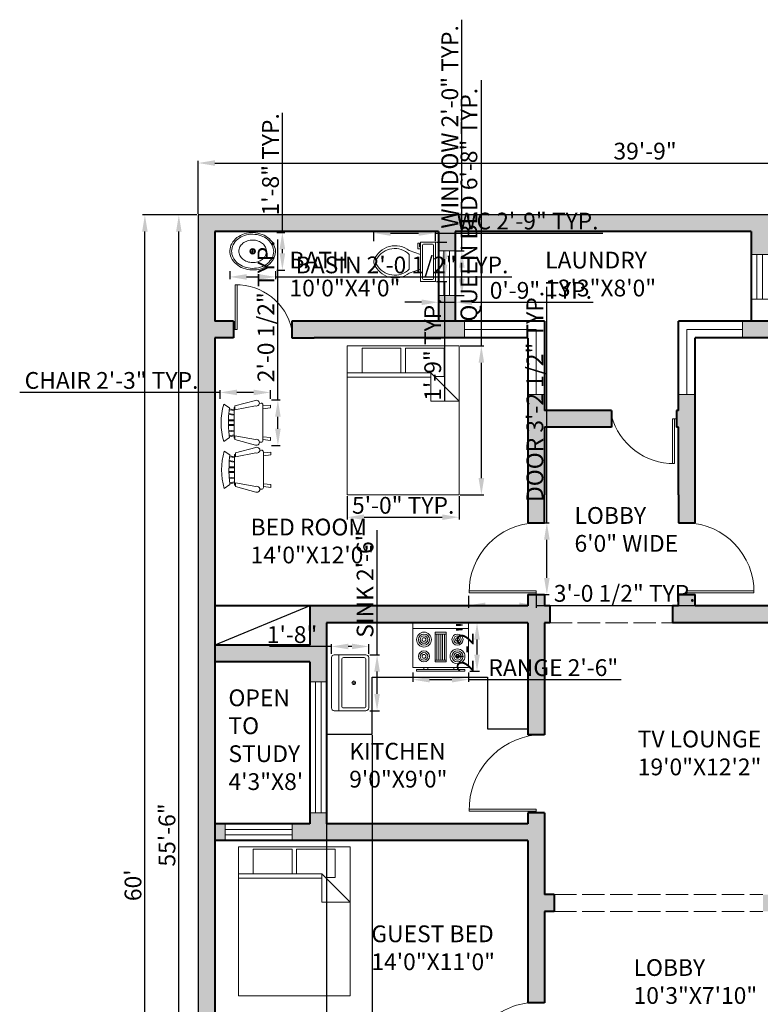
# Model space of a CAD drawing. Units: inches. Extents: x 1967493 to 1968177, y 907234 to 908105.
# Tile 4 of 5: x 1967493 to 1967891, y 907576 to 908105. Entities that reach past the tile are written whole.
import ezdxf

# ---------------------------------------------------------------- set-up
doc = ezdxf.new("R2010")
doc.units = ezdxf.units.IN
doc.linetypes.add('ACAD_ISO02W100', pattern=[15, 12, -3])
for name, color, linetype, lineweight in [('A-ANNO-DIMS', 2, 'Continuous', 18), ('A-AREA-IDEN', 7, 'Continuous', 25), ('A-DOOR', 3, 'Continuous', 20), ('A-EQPM', 8, 'Continuous', 20), ('A-FLOR-CASE', 9, 'Continuous', 25), ('A-FLOR-FIXT', 9, 'Continuous', 18), ('A-FURN', 8, 'Continuous', 18), ('A-GLAZ', 4, 'Continuous', 18), ('A-WALL', 7, 'Continuous', 40), ('A-WALL-OVHD', 7, 'ACAD_ISO02W100', 18), ('C-PROP', 7, 'Continuous', 25)]:
    doc.layers.add(name, color=color, linetype=linetype, lineweight=lineweight)
doc.layers.add('A-WALL-PATT', color=18, linetype='Continuous', lineweight=13, true_color=0x000000)
doc.styles.get("Standard").update_dxf_attribs({"font": 'arial.ttf'})
doc.dimstyles.new('ISO-25', dxfattribs={"dimtxt": 9, "dimasz": 9, "dimexe": 1.25, "dimexo": 0.625, "dimtad": 1, "dimdec": 1, "dimrnd": 9, "dimlunit": 3, "dimtxsty": 'Standard', "dimcen": 2.5, "dimadec": 0, "dimazin": 0, "dimtfac": 1, "dimtdec": 1, "dimtmove": 0, "dimatfit": 3, "dimfxl": 1, "dimarcsym": 0})

# ---------------------------------------------------------------- blocks, each defined once
blk = doc.blocks.new('Bed - Queen')
for p, q in [((0, -80.00003), (0, 0)), ((0, 0), (59.99999, 0)), ((59.99999, 0), (59.99999, -80.00003)), ((7.99999, -1.2), (28.79998, -1.2)), ((7.99999, -14.4), (7.99999, -1.2)), ((28.79998, -1.2), (28.79998, -14.4)), ((31.19999, -1.2), (51.99999, -1.2)), ((31.19999, -14.4), (31.19999, -1.2)), ((51.99999, -1.2), (51.99999, -16.4)), ((0, -14.4), (44.8, -14.4)), ((59.99999, -29.6), (44.8, -14.4)), ((44.8, -14.4), (44.8, -29.6)), ((44.8, -16.8), (0, -16.8)), ((51.99999, -16.4), (46.79936, -16.4)), ((44.8, -29.6), (59.99999, -29.6)), ((59.99999, -80.00003), (0, -80.00003))]:
    blk.add_line(p, q)
blk = doc.blocks.new('Sink - Oval top')
for p, q in [((-1, 0), (1, 0)), ((0, 1), (0, -1))]:
    blk.add_line(p, q)
for points in [[(-12.23, 0.39, 0.117634), (-11.46, -3.36, 0.104469), (-8.88, -6.8, 0.090016), (-5.08, -9.07, 0.08192), (-0.32, -10.02, 0.08192), (4.49, -9.38, 0.090016), (8.42, -7.36, 0.104469), (11.22, -4.09, 0.117634), (12.23, -0.39, 0.117634), (11.46, 3.36, 0.104469), (8.88, 6.8, 0.090016), (5.08, 9.07, 0.08192), (0.32, 10.02, 0.08192), (-4.49, 9.38, 0.090016), (-8.42, 7.36, 0.104469), (-11.22, 4.09, 0.117634)], [(-11.29, 0.16, 0.118622), (-10.52, -3.25, 0.104678), (-8.07, -6.36, 0.089562), (-4.54, -8.37, 0.081185), (-0.13, -9.15, 0.081185), (4.3, -8.49, 0.089562), (7.89, -6.58, 0.104678), (10.42, -3.55, 0.118622), (11.29, -0.16, 0.118622), (10.52, 3.25, 0.104678), (8.07, 6.36, 0.089562), (4.54, 8.37, 0.081185), (0.13, 9.15, 0.081185), (-4.3, 8.49, 0.089562), (-7.89, 6.58, 0.104678), (-10.42, 3.55, 0.118622)], [(-7.42, 0.08, 0.118283), (-6.91, -2.17, 0.104607), (-5.29, -4.21, 0.089718), (-2.97, -5.53, 0.081436), (-0.07, -6.04, 0.081436), (2.84, -5.59, 0.089718), (5.2, -4.33, 0.104607), (6.86, -2.32, 0.118283), (7.42, -0.08, 0.118283), (6.91, 2.17, 0.104607), (5.29, 4.21, 0.089718), (2.97, 5.53, 0.081436), (0.07, 6.04, 0.081436), (-2.84, 5.59, 0.089718), (-5.2, 4.33, 0.104607), (-6.86, 2.32, 0.118283)]]:
    blk.add_lwpolyline(points, format="xyb", close=True)
for radius in [1.5, 1]:
    blk.add_circle((0, 0), radius)
blk = doc.blocks.new('Range-Oven - 30 in top')
for p, q in [((0, -3), (30, -3)), ((12, -6), (18, -6)), ((13, -20), (13, -6)), ((14, -6), (14, -20)), ((15, -20), (15, -6)), ((16, -6), (16, -20)), ((17, -20), (17, -6)), ((18, -20), (12, -20)), ((6, -24), (6, -25)), ((8, -25), (8, -24)), ((22, -25), (22, -24)), ((24, -24), (24, -25))]:
    blk.add_line(p, q)
for points in [[(0, -24), (0, 0), (30, 0), (30, -24)], [(12, -21), (12, -5), (18, -5), (18, -21)], [(2, -26), (2, -25), (28, -25), (28, -26)]]:
    blk.add_lwpolyline(points, close=True)
for centre, radius in [((6, -9), 4), ((6, -9), 3), ((6, -9), 2), ((6, -9), 1), ((24, -9), 3), ((24, -9), 2), ((24, -9), 1), ((6, -18), 3), ((24, -18), 4), ((24, -18), 3), ((6, -18), 2), ((6, -18), 1), ((24, -18), 2), ((24, -18), 1)]:
    blk.add_circle(centre, radius)
blk = doc.blocks.new('Sink-single - 30 in top')
blk.add_line((-15, -3.999996), (15, -3.999996))
for points in [[(-13.5, 0), (13.5, 0)], [(-15, -18.499996), (-15, -1.5)], [(15, -1.5), (15, -18.499996)], [(-13.5, -17.499996), (-13.5, -6.499996)], [(-12.5, -5.499996), (12.5, -5.499996)], [(13.5, -6.499996), (13.5, -17.499996)], [(13.5, -19.999996), (-13.5, -19.999996)], [(12.5, -18.499996), (-12.5, -18.499996)]]:
    blk.add_lwpolyline(points)
for radius in [1, 0.5]:
    blk.add_circle((0, -11.999996), radius)
for centre, radius, start, end in [((-13.5, -1.5), 1.5, 90, 180), ((13.5, -1.5), 1.5, 0, 90), ((-12.5, -6.499996), 1, 90, 180), ((12.5, -6.499996), 1, 0, 90), ((-13.5, -18.499996), 1.5, 180, 270), ((-12.5, -17.499996), 1, 180, 270), ((12.5, -17.499996), 1, 270, 0), ((13.5, -18.499996), 1.5, 270, 0)]:
    blk.add_arc(centre, radius, start, end)
blk = doc.blocks.new('Toilet - top')
for p, q in [((9.5, -6), (9.5, -2)), ((-10, -8.5), (-8, -8.5)), ((-10, -9.5), (-10, -8.5)), ((-7, -9.5), (-10, -9.5)), ((-8, -8.5), (-8, -8)), ((-7, -8), (-7, -9.5)), ((-4, -8), (-6, -14)), ((4, -8), (6, -14)), ((4, -14), (-4, -14))]:
    blk.add_line(p, q)
blk.add_lwpolyline([(10.5, -8), (10.5, 0), (-10.5, 0), (-10.5, -8)], close=True)
for points in [[(-9.5, -2), (-9.5, -6)], [(8.5, -1), (-8.5, -1)], [(-8.5, -7), (8.5, -7)]]:
    blk.add_lwpolyline(points)
for centre, radius, start, end in [((-8.62, -1.88), 0.884, 81.8699, 188.1301), ((8.62, -1.88), 0.884, 351.8699, 98.1301), ((-8.62, -6.12), 0.884, 171.8699, 278.1301), ((8.62, -6.12), 0.884, 261.8699, 8.1301), ((3.52, -21.58), 12.17, 141.4691, 247.9714), ((4.2, -21.82), 11.33, 136.3677, 238.9468), ((-3.52, -21.58), 12.17, 292.0284, 38.5307), ((-4.2, -21.82), 11.33, 301.053, 43.6321), ((0, -27.88), 4, 245.7318, 294.2682), ((0, -29), 4, 254.8605, 285.1395)]:
    blk.add_arc(centre, radius, start, end)
blk = doc.blocks.new('Chair - Rocking')
for p, q in [((-8, -4.5), (-10, -1.5)), ((-7.5, -4.5), (-7, -7)), ((-6.5, -7), (-7.02225, -4.43)), ((-4.5, -7), (-4.96674, -4.19951)), ((-4, -7), (-4.40532, -4.16272)), ((-1.5, -4.05012), (-1.5, -7)), ((-1, -7), (-1, -4.05012)), ((1, -7), (1, -4.04655)), ((1.5, -4.05012), (1.5, -7)), ((4, -7), (4.40187, -4.18694)), ((4.5, -7), (4.96761, -4.19437)), ((6.5, -7), (7, -4.4057)), ((7.5, -4.5), (7, -7)), ((8, -4.5), (10, -1.5)), ((-9, -7.5), (-12, -18.49999)), ((-7, -7.5), (-9, -7.5)), ((-9, -18.49999), (-7, -7.5)), ((-8.23428, -6.99939), (-8.3093, -7.47958)), ((-8.23041, -7), (8.23915, -7)), ((7, -7.5), (9, -7.5)), ((9, -18.49999), (7, -7.5)), ((8.31071, -7.48854), (8.23449, -7.00073)), ((9, -7.5), (12, -18.49999)), ((-10.36644, -20.64523), (-10.5, -21.49999)), ((10.5, -21.49999), (10.3575, -20.58798)), ((-9, -22.49999), (-9.5, -26.49999)), ((0, -22.49999), (-9.5, -22.49999)), ((-8, -26.49999), (-7.5, -22.49999)), ((0, -22.49999), (9.5, -22.49999)), ((8, -26.49999), (7.5, -22.49999)), ((9, -22.49999), (9.5, -26.49999)), ((-9.5, -26.49999), (-8, -26.49999)), ((9.5, -26.49999), (8, -26.49999))]:
    blk.add_line(p, q)
for centre, radius, start, end in [((0, -34.08333), 34.08333, 72.93847, 107.0615), ((0, -68.25004), 64.25, 93.92211, 97.15267), ((0, -68.25004), 64.25, 82.84733, 93.92211), ((-10.5, -18.99999), 1.58114, 161.5651, 18.43495), ((10.5, -18.99999), 1.58114, 161.5651, 18.43495), ((-9.5, -21.49999), 1, 180, 270), ((9.5, -21.49999), 1, 270, 0)]:
    blk.add_arc(centre, radius, start, end)
blk = doc.blocks.new('*D11')
at = {"layer": 'A-ANNO-DIMS', "color": 0, "lineweight": -2, "transparency": 16777216}
for p, q in [((1967588.78, 908000.79), (1967588.78, 908029.28)), ((1967597.78, 908028.03), (1968059.78, 908028.03)), ((1968068.78, 908000.79), (1968068.78, 908029.28))]:
    blk.add_line(p, q, dxfattribs=at)
at = {"layer": 'A-ANNO-DIMS', "color": 0, "transparency": 16777216}
for points in [[(1967597.78, 908029.53), (1967597.78, 908026.53), (1967588.78, 908028.03)], [(1968059.78, 908029.53), (1968059.78, 908026.53), (1968068.78, 908028.03)]]:
    blk.add_solid(points, dxfattribs=at)
at = {"layer": 'Defpoints', "color": 0, "transparency": 16777216}
for p in [(1968068.78, 908028.03), (1967588.78, 908000.17), (1968068.78, 908000.17)]:
    blk.add_point(p, dxfattribs=at)
at = {"layer": 'A-ANNO-DIMS', "color": 0, "transparency": 16777216, "insert": (1967828.78, 908033.25), "char_height": 9, "attachment_point": 5}
blk.add_mtext('39\'-9"', dxfattribs=at)
blk = doc.blocks.new('*D12')
at = {"layer": 'A-ANNO-DIMS', "color": 0, "lineweight": -2, "transparency": 16777216}
for p, q in [((1967588.15, 908000.17), (1967558.93, 908000.17)), ((1967560.18, 907289.17), (1967560.18, 907991.17)), ((1967588.15, 907280.17), (1967558.93, 907280.17))]:
    blk.add_line(p, q, dxfattribs=at)
at = {"layer": 'A-ANNO-DIMS', "color": 0, "transparency": 16777216}
for points in [[(1967558.68, 907991.17), (1967561.68, 907991.17), (1967560.18, 908000.17)], [(1967558.68, 907289.17), (1967561.68, 907289.17), (1967560.18, 907280.17)]]:
    blk.add_solid(points, dxfattribs=at)
at = {"layer": 'Defpoints', "color": 0, "transparency": 16777216}
for p in [(1967560.18, 908000.17), (1967588.78, 908000.17), (1967588.78, 907280.17)]:
    blk.add_point(p, dxfattribs=at)
at = {"layer": 'A-ANNO-DIMS', "color": 0, "transparency": 16777216, "insert": (1967554.96, 907640.17), "char_height": 9, "attachment_point": 5, "rotation": 90}
blk.add_mtext("60'", dxfattribs=at)
blk = doc.blocks.new('*D13')
at = {"layer": 'A-ANNO-DIMS', "color": 0, "lineweight": -2, "transparency": 16777216}
for p, q in [((1967588.15, 908000.17), (1967577.16, 908000.17)), ((1967578.41, 907343.17), (1967578.41, 907991.17)), ((1967588.15, 907334.17), (1967577.16, 907334.17))]:
    blk.add_line(p, q, dxfattribs=at)
at = {"layer": 'A-ANNO-DIMS', "color": 0, "transparency": 16777216}
for points in [[(1967576.91, 907991.17), (1967579.91, 907991.17), (1967578.41, 908000.17)], [(1967576.91, 907343.17), (1967579.91, 907343.17), (1967578.41, 907334.17)]]:
    blk.add_solid(points, dxfattribs=at)
at = {"layer": 'Defpoints', "color": 0, "transparency": 16777216}
for p in [(1967578.41, 908000.17), (1967588.78, 908000.17), (1967588.78, 907334.17)]:
    blk.add_point(p, dxfattribs=at)
at = {"layer": 'A-ANNO-DIMS', "color": 0, "transparency": 16777216, "insert": (1967573.19, 907667.17), "char_height": 9, "attachment_point": 5, "rotation": 90}
blk.add_mtext('55\'-6"', dxfattribs=at)
blk = doc.blocks.new('WIN-36IN')
for p, q in [((0, 9), (0, 0)), ((36, 6), (0, 6)), ((36, 9), (36, 0)), ((36, 3), (0, 3))]:
    blk.add_line(p, q)
blk = doc.blocks.new('DOOR-SINGLE-36IN')
for p, q in [((0, 1), (0, 2)), ((0, 2), (36, 2)), ((36, 1), (0, 1)), ((36, 2), (36, 1)), ((36, 0), (36, 1))]:
    blk.add_line(p, q)
blk.add_arc((37.01, 1.5), 37.01, 91.5627, 180.774)
blk = doc.blocks.new('WIN-24IN')
for p, q in [((0, 24), (9, 24)), ((3, 24), (3, 0)), ((6, 24), (6, 0)), ((0, 0), (9, 0))]:
    blk.add_line(p, q)
blk = doc.blocks.new('*D18')
at = {"layer": 'A-ANNO-DIMS', "color": 0, "lineweight": -2, "transparency": 16777216}
for p, q in [((1967600.56, 907904.83), (1967492.95, 907904.83)), ((1967600.56, 907901.4), (1967600.56, 907906.08)), ((1967618.56, 907904.83), (1967609.56, 907904.83)), ((1967627.56, 907901.4), (1967627.56, 907906.08))]:
    blk.add_line(p, q, dxfattribs=at)
at = {"layer": 'A-ANNO-DIMS', "color": 0, "transparency": 16777216}
for points in [[(1967609.56, 907906.33), (1967609.56, 907903.33), (1967600.56, 907904.83)], [(1967618.56, 907906.33), (1967618.56, 907903.33), (1967627.56, 907904.83)]]:
    blk.add_solid(points, dxfattribs=at)
at = {"layer": 'Defpoints', "color": 0, "transparency": 16777216}
for p in [(1967600.56, 907904.83), (1967600.56, 907900.78), (1967627.56, 907900.78)]:
    blk.add_point(p, dxfattribs=at)
at = {"layer": 'A-ANNO-DIMS', "color": 0, "transparency": 16777216, "insert": (1967542.26, 907910.11), "char_height": 9, "attachment_point": 5}
blk.add_mtext('CHAIR 2\'-3" TYP.', dxfattribs=at)
blk = doc.blocks.new('*D19')
at = {"layer": 'A-ANNO-DIMS', "color": 0, "lineweight": -2, "transparency": 16777216}
for p, q in [((1967631.61, 907900.78), (1967631.61, 907987.01)), ((1967628.19, 907900.78), (1967632.86, 907900.78)), ((1967631.61, 907885.34), (1967631.61, 907891.78)), ((1967628.19, 907876.34), (1967632.86, 907876.34))]:
    blk.add_line(p, q, dxfattribs=at)
at = {"layer": 'A-ANNO-DIMS', "color": 0, "transparency": 16777216}
for points in [[(1967630.11, 907891.78), (1967633.11, 907891.78), (1967631.61, 907900.78)], [(1967630.11, 907885.34), (1967633.11, 907885.34), (1967631.61, 907876.34)]]:
    blk.add_solid(points, dxfattribs=at)
at = {"layer": 'Defpoints', "color": 0, "transparency": 16777216}
for p in [(1967627.56, 907900.78), (1967631.61, 907900.78), (1967627.56, 907876.34)]:
    blk.add_point(p, dxfattribs=at)
at = {"layer": 'A-ANNO-DIMS', "color": 0, "transparency": 16777216, "insert": (1967626.34, 907948.39), "char_height": 9, "attachment_point": 5, "rotation": 90}
blk.add_mtext('2\'-0 1/2" TYP.', dxfattribs=at)
blk = doc.blocks.new('*D24')
at = {"layer": 'A-ANNO-DIMS', "color": 0, "lineweight": -2, "transparency": 16777216}
for p, q in [((1967740.89, 907929.81), (1967740.89, 908072.45)), ((1967729.52, 907929.81), (1967742.14, 907929.81)), ((1967740.89, 907858.81), (1967740.89, 907920.81)), ((1967729.52, 907849.81), (1967742.14, 907849.81))]:
    blk.add_line(p, q, dxfattribs=at)
at = {"layer": 'A-ANNO-DIMS', "color": 0, "transparency": 16777216}
for points in [[(1967739.39, 907920.81), (1967742.39, 907920.81), (1967740.89, 907929.81)], [(1967739.39, 907858.81), (1967742.39, 907858.81), (1967740.89, 907849.81)]]:
    blk.add_solid(points, dxfattribs=at)
at = {"layer": 'Defpoints', "color": 0, "transparency": 16777216}
for p in [(1967728.89, 907929.81), (1967740.89, 907929.81), (1967728.89, 907849.81)]:
    blk.add_point(p, dxfattribs=at)
at = {"layer": 'A-ANNO-DIMS', "color": 0, "transparency": 16777216, "insert": (1967735.34, 908005.63), "char_height": 9, "attachment_point": 5, "rotation": 90}
blk.add_mtext('QUEEN BED 6\'-8" TYP.', dxfattribs=at)
blk = doc.blocks.new('*D25')
at = {"layer": 'A-ANNO-DIMS', "color": 0, "lineweight": -2, "transparency": 16777216}
for p, q in [((1967668.89, 907849.18), (1967668.89, 907836.56)), ((1967728.89, 907849.18), (1967728.89, 907836.56)), ((1967677.89, 907837.81), (1967719.89, 907837.81))]:
    blk.add_line(p, q, dxfattribs=at)
at = {"layer": 'A-ANNO-DIMS', "color": 0, "transparency": 16777216}
for points in [[(1967677.89, 907839.31), (1967677.89, 907836.31), (1967668.89, 907837.81)], [(1967719.89, 907839.31), (1967719.89, 907836.31), (1967728.89, 907837.81)]]:
    blk.add_solid(points, dxfattribs=at)
at = {"layer": 'Defpoints', "color": 0, "transparency": 16777216}
for p in [(1967668.89, 907849.81), (1967728.89, 907849.81), (1967728.89, 907837.81)]:
    blk.add_point(p, dxfattribs=at)
at = {"layer": 'A-ANNO-DIMS', "color": 0, "transparency": 16777216, "insert": (1967698.89, 907843.03), "char_height": 9, "attachment_point": 5}
blk.add_mtext('5\'-0" TYP.', dxfattribs=at)
blk = doc.blocks.new('*D26')
at = {"layer": 'A-ANNO-DIMS', "color": 0, "lineweight": -2, "transparency": 16777216}
for p, q in [((1967683.13, 907986.09), (1967683.13, 907991.67)), ((1967692.13, 907990.42), (1967707.18, 907990.42)), ((1967716.18, 907986.09), (1967716.18, 907991.67)), ((1967716.18, 907990.42), (1967806.1, 907990.42))]:
    blk.add_line(p, q, dxfattribs=at)
at = {"layer": 'A-ANNO-DIMS', "color": 0, "transparency": 16777216}
for points in [[(1967692.13, 907991.92), (1967692.13, 907988.92), (1967683.13, 907990.42)], [(1967707.18, 907991.92), (1967707.18, 907988.92), (1967716.18, 907990.42)]]:
    blk.add_solid(points, dxfattribs=at)
at = {"layer": 'Defpoints', "color": 0, "transparency": 16777216}
for p in [(1967716.18, 907990.42), (1967683.13, 907985.46), (1967716.18, 907985.46)]:
    blk.add_point(p, dxfattribs=at)
at = {"layer": 'A-ANNO-DIMS', "color": 0, "transparency": 16777216, "insert": (1967765.64, 907995.7), "char_height": 9, "attachment_point": 5}
blk.add_mtext('WC 2\'-9" TYP.', dxfattribs=at)
blk = doc.blocks.new('*D27')
at = {"layer": 'A-ANNO-DIMS', "color": 0, "lineweight": -2, "transparency": 16777216}
for p, q in [((1967716.8, 907985.46), (1967722.39, 907985.46)), ((1967721.14, 907976.46), (1967721.14, 907973.46)), ((1967716.8, 907964.46), (1967722.39, 907964.46)), ((1967721.14, 907964.46), (1967721.14, 907900.2))]:
    blk.add_line(p, q, dxfattribs=at)
at = {"layer": 'A-ANNO-DIMS', "color": 0, "transparency": 16777216}
for points in [[(1967719.64, 907976.46), (1967722.64, 907976.46), (1967721.14, 907985.46)], [(1967719.64, 907973.46), (1967722.64, 907973.46), (1967721.14, 907964.46)]]:
    blk.add_solid(points, dxfattribs=at)
at = {"layer": 'Defpoints', "color": 0, "transparency": 16777216}
for p in [(1967716.18, 907985.46), (1967716.18, 907964.46), (1967721.14, 907964.46)]:
    blk.add_point(p, dxfattribs=at)
at = {"layer": 'A-ANNO-DIMS', "color": 0, "transparency": 16777216, "insert": (1967715.92, 907927.83), "char_height": 9, "attachment_point": 5, "rotation": 90}
blk.add_mtext('1\'-9" TYP.', dxfattribs=at)
blk = doc.blocks.new('*D28')
at = {"layer": 'A-ANNO-DIMS', "color": 0, "lineweight": -2, "transparency": 16777216}
for p, q in [((1967605.78, 907969.92), (1967605.78, 907965.61)), ((1967630.33, 907969.92), (1967630.33, 907965.61)), ((1967614.78, 907966.86), (1967621.33, 907966.86)), ((1967630.33, 907966.86), (1967757.24, 907966.86))]:
    blk.add_line(p, q, dxfattribs=at)
at = {"layer": 'A-ANNO-DIMS', "color": 0, "transparency": 16777216}
for points in [[(1967614.78, 907968.36), (1967614.78, 907965.36), (1967605.78, 907966.86)], [(1967621.33, 907968.36), (1967621.33, 907965.36), (1967630.33, 907966.86)]]:
    blk.add_solid(points, dxfattribs=at)
at = {"layer": 'Defpoints', "color": 0, "transparency": 16777216}
for p in [(1967605.78, 907970.55), (1967630.33, 907970.55), (1967630.33, 907966.86)]:
    blk.add_point(p, dxfattribs=at)
at = {"layer": 'A-ANNO-DIMS', "color": 0, "transparency": 16777216, "insert": (1967698.28, 907972.14), "char_height": 9, "attachment_point": 5}
blk.add_mtext('BASIN 2\'-0 1/2" TYP.', dxfattribs=at)
blk = doc.blocks.new('*D29')
at = {"layer": 'A-ANNO-DIMS', "color": 0, "lineweight": -2, "transparency": 16777216}
for p, q in [((1967634.01, 907990.68), (1967634.01, 908054.95)), ((1967630.96, 907990.68), (1967635.26, 907990.68)), ((1967634.01, 907979.55), (1967634.01, 907981.68)), ((1967630.96, 907970.55), (1967635.26, 907970.55))]:
    blk.add_line(p, q, dxfattribs=at)
at = {"layer": 'A-ANNO-DIMS', "color": 0, "transparency": 16777216}
for points in [[(1967632.51, 907981.68), (1967635.51, 907981.68), (1967634.01, 907990.68)], [(1967632.51, 907979.55), (1967635.51, 907979.55), (1967634.01, 907970.55)]]:
    blk.add_solid(points, dxfattribs=at)
at = {"layer": 'Defpoints', "color": 0, "transparency": 16777216}
for p in [(1967630.33, 907990.68), (1967634.01, 907990.68), (1967630.33, 907970.55)]:
    blk.add_point(p, dxfattribs=at)
at = {"layer": 'A-ANNO-DIMS', "color": 0, "transparency": 16777216, "insert": (1967628.79, 908027.31), "char_height": 9, "attachment_point": 5, "rotation": 90}
blk.add_mtext('1\'-8" TYP.', dxfattribs=at)
blk = doc.blocks.new('*D34')
at = {"layer": 'A-ANNO-DIMS', "color": 0, "lineweight": -2, "transparency": 16777216}
for p, q in [((1967776.05, 907834.76), (1967776.05, 907961.6)), ((1967770.9, 907834.76), (1967777.3, 907834.76)), ((1967776.05, 907805.26), (1967776.05, 907825.76)), ((1967770.9, 907796.26), (1967777.3, 907796.26))]:
    blk.add_line(p, q, dxfattribs=at)
at = {"layer": 'A-ANNO-DIMS', "color": 0, "transparency": 16777216}
for points in [[(1967774.55, 907825.76), (1967777.55, 907825.76), (1967776.05, 907834.76)], [(1967774.55, 907805.26), (1967777.55, 907805.26), (1967776.05, 907796.26)]]:
    blk.add_solid(points, dxfattribs=at)
at = {"layer": 'Defpoints', "color": 0, "transparency": 16777216}
for p in [(1967770.28, 907834.76), (1967776.05, 907834.76), (1967770.28, 907796.26)]:
    blk.add_point(p, dxfattribs=at)
at = {"layer": 'A-ANNO-DIMS', "color": 0, "transparency": 16777216, "insert": (1967770.77, 907902.68), "char_height": 9, "attachment_point": 5, "rotation": 90}
blk.add_mtext('DOOR 3\'-2 1/2" TYP.', dxfattribs=at)
blk = doc.blocks.new('*D35')
at = {"layer": 'A-ANNO-DIMS', "color": 0, "lineweight": -2, "transparency": 16777216}
for p, q in [((1967734.01, 907795.64), (1967734.01, 907789.24)), ((1967770.28, 907795.64), (1967770.28, 907789.24)), ((1967743.01, 907790.49), (1967761.28, 907790.49)), ((1967770.28, 907790.49), (1967856.35, 907790.49))]:
    blk.add_line(p, q, dxfattribs=at)
at = {"layer": 'A-ANNO-DIMS', "color": 0, "transparency": 16777216}
for points in [[(1967743.01, 907791.99), (1967743.01, 907788.99), (1967734.01, 907790.49)], [(1967761.28, 907791.99), (1967761.28, 907788.99), (1967770.28, 907790.49)]]:
    blk.add_solid(points, dxfattribs=at)
at = {"layer": 'Defpoints', "color": 0, "transparency": 16777216}
for p in [(1967734.01, 907796.26), (1967770.28, 907796.26), (1967770.28, 907790.49)]:
    blk.add_point(p, dxfattribs=at)
at = {"layer": 'A-ANNO-DIMS', "color": 0, "transparency": 16777216, "insert": (1967817.82, 907795.77), "char_height": 9, "attachment_point": 5}
blk.add_mtext('3\'-0 1/2" TYP.', dxfattribs=at)
blk = doc.blocks.new('*D36')
at = {"layer": 'A-ANNO-DIMS', "color": 0, "lineweight": -2, "transparency": 16777216}
for p, q in [((1967730.38, 907980.85), (1967730.38, 908104.99)), ((1967727.4, 907980.85), (1967731.63, 907980.85)), ((1967730.38, 907965.85), (1967730.38, 907971.85)), ((1967727.4, 907956.85), (1967731.63, 907956.85))]:
    blk.add_line(p, q, dxfattribs=at)
at = {"layer": 'A-ANNO-DIMS', "color": 0, "transparency": 16777216}
for points in [[(1967728.88, 907971.85), (1967731.88, 907971.85), (1967730.38, 907980.85)], [(1967728.88, 907965.85), (1967731.88, 907965.85), (1967730.38, 907956.85)]]:
    blk.add_solid(points, dxfattribs=at)
at = {"layer": 'Defpoints', "color": 0, "transparency": 16777216}
for p in [(1967726.78, 907980.85), (1967730.38, 907980.85), (1967726.78, 907956.85)]:
    blk.add_point(p, dxfattribs=at)
at = {"layer": 'A-ANNO-DIMS', "color": 0, "transparency": 16777216, "insert": (1967725.1, 908047.42), "char_height": 9, "attachment_point": 5, "rotation": 90}
blk.add_mtext('WINDOW 2\'-0" TYP.', dxfattribs=at)
blk = doc.blocks.new('*D37')
at = {"layer": 'A-ANNO-DIMS', "color": 0, "lineweight": -2, "transparency": 16777216}
for p, q in [((1967708.78, 907953.25), (1967699.78, 907953.25)), ((1967717.78, 907956.23), (1967717.78, 907952)), ((1967717.78, 907953.25), (1967726.78, 907953.25)), ((1967726.78, 907956.23), (1967726.78, 907952)), ((1967735.78, 907953.25), (1967800.89, 907953.25))]:
    blk.add_line(p, q, dxfattribs=at)
at = {"layer": 'A-ANNO-DIMS', "color": 0, "transparency": 16777216}
for points in [[(1967708.78, 907954.75), (1967708.78, 907951.75), (1967717.78, 907953.25)], [(1967735.78, 907954.75), (1967735.78, 907951.75), (1967726.78, 907953.25)]]:
    blk.add_solid(points, dxfattribs=at)
at = {"layer": 'Defpoints', "color": 0, "transparency": 16777216}
for p in [(1967717.78, 907956.85), (1967726.78, 907956.85), (1967726.78, 907953.25)]:
    blk.add_point(p, dxfattribs=at)
at = {"layer": 'A-ANNO-DIMS', "color": 0, "transparency": 16777216, "insert": (1967772.83, 907958.47), "char_height": 9, "attachment_point": 5}
blk.add_mtext('0\'-9" TYP.', dxfattribs=at)
blk = doc.blocks.new('*D40')
at = {"layer": 'A-ANNO-DIMS', "color": 0, "lineweight": -2, "transparency": 16777216}
for p, q in [((1967704.05, 907754.46), (1967704.05, 907749.34)), ((1967734.05, 907754.46), (1967734.05, 907749.34)), ((1967713.05, 907750.59), (1967725.05, 907750.59)), ((1967734.05, 907750.59), (1967815.97, 907750.59))]:
    blk.add_line(p, q, dxfattribs=at)
at = {"layer": 'A-ANNO-DIMS', "color": 0, "transparency": 16777216}
for points in [[(1967713.05, 907752.09), (1967713.05, 907749.09), (1967704.05, 907750.59)], [(1967725.05, 907752.09), (1967725.05, 907749.09), (1967734.05, 907750.59)]]:
    blk.add_solid(points, dxfattribs=at)
at = {"layer": 'Defpoints', "color": 0, "transparency": 16777216}
for p in [(1967704.05, 907755.09), (1967734.05, 907755.09), (1967734.05, 907750.59)]:
    blk.add_point(p, dxfattribs=at)
at = {"layer": 'A-ANNO-DIMS', "color": 0, "transparency": 16777216, "insert": (1967779.51, 907755.87), "char_height": 9, "attachment_point": 5}
blk.add_mtext('RANGE 2\'-6"', dxfattribs=at)
blk = doc.blocks.new('*D41')
at = {"layer": 'A-ANNO-DIMS', "color": 0, "lineweight": -2, "transparency": 16777216}
for p, q in [((1967734.68, 907781.09), (1967739.8, 907781.09)), ((1967738.55, 907764.09), (1967738.55, 907772.09)), ((1967734.68, 907755.09), (1967739.8, 907755.09))]:
    blk.add_line(p, q, dxfattribs=at)
at = {"layer": 'A-ANNO-DIMS', "color": 0, "transparency": 16777216}
for points in [[(1967737.05, 907772.09), (1967740.05, 907772.09), (1967738.55, 907781.09)], [(1967737.05, 907764.09), (1967740.05, 907764.09), (1967738.55, 907755.09)]]:
    blk.add_solid(points, dxfattribs=at)
at = {"layer": 'Defpoints', "color": 0, "transparency": 16777216}
for p in [(1967734.05, 907781.09), (1967738.55, 907781.09), (1967734.05, 907755.09)]:
    blk.add_point(p, dxfattribs=at)
at = {"layer": 'A-ANNO-DIMS', "color": 0, "transparency": 16777216, "insert": (1967733.41, 907768.09), "char_height": 9, "attachment_point": 5, "rotation": 90}
blk.add_mtext('2\'-2"', dxfattribs=at)
blk = doc.blocks.new('*D42')
at = {"layer": 'A-ANNO-DIMS', "color": 0, "lineweight": -2, "transparency": 16777216}
for p, q in [((1967684.87, 907763.91), (1967684.87, 907830.88)), ((1967680.99, 907763.91), (1967686.12, 907763.91)), ((1967684.87, 907742.91), (1967684.87, 907754.91)), ((1967680.99, 907733.91), (1967686.12, 907733.91))]:
    blk.add_line(p, q, dxfattribs=at)
at = {"layer": 'A-ANNO-DIMS', "color": 0, "transparency": 16777216}
for points in [[(1967683.37, 907754.91), (1967686.37, 907754.91), (1967684.87, 907763.91)], [(1967683.37, 907742.91), (1967686.37, 907742.91), (1967684.87, 907733.91)]]:
    blk.add_solid(points, dxfattribs=at)
at = {"layer": 'Defpoints', "color": 0, "transparency": 16777216}
for p in [(1967680.37, 907763.91), (1967684.87, 907763.91), (1967680.37, 907733.91)]:
    blk.add_point(p, dxfattribs=at)
at = {"layer": 'A-ANNO-DIMS', "color": 0, "transparency": 16777216, "insert": (1967679.59, 907801.89), "char_height": 9, "attachment_point": 5, "rotation": 90}
blk.add_mtext('SINK 2\'-6"', dxfattribs=at)
blk = doc.blocks.new('*D43')
at = {"layer": 'A-ANNO-DIMS', "color": 0, "lineweight": -2, "transparency": 16777216}
for p, q in [((1967660.37, 907768.41), (1967627.04, 907768.41)), ((1967660.37, 907764.53), (1967660.37, 907769.66)), ((1967671.37, 907768.41), (1967669.37, 907768.41)), ((1967680.37, 907764.53), (1967680.37, 907769.66))]:
    blk.add_line(p, q, dxfattribs=at)
at = {"layer": 'A-ANNO-DIMS', "color": 0, "transparency": 16777216}
for points in [[(1967669.37, 907769.91), (1967669.37, 907766.91), (1967660.37, 907768.41)], [(1967671.37, 907769.91), (1967671.37, 907766.91), (1967680.37, 907768.41)]]:
    blk.add_solid(points, dxfattribs=at)
at = {"layer": 'Defpoints', "color": 0, "transparency": 16777216}
for p in [(1967660.37, 907768.41), (1967660.37, 907763.91), (1967680.37, 907763.91)]:
    blk.add_point(p, dxfattribs=at)
at = {"layer": 'A-ANNO-DIMS', "color": 0, "transparency": 16777216, "insert": (1967639.2, 907773.63), "char_height": 9, "attachment_point": 5}
blk.add_mtext('1\'-8"', dxfattribs=at)
blk = doc.blocks.new('*D52')
at = {"layer": 'A-ANNO-DIMS', "color": 0, "lineweight": -2, "transparency": 16777216}
for p, q in [((1967657.78, 907720.78), (1967657.78, 907240.77)), ((1967682.26, 907720.78), (1967682.26, 907240.77)), ((1967666.78, 907242.02), (1967673.26, 907242.02)), ((1967682.26, 907242.02), (1967737.56, 907242.02))]:
    blk.add_line(p, q, dxfattribs=at)
at = {"layer": 'A-ANNO-DIMS', "color": 0, "transparency": 16777216}
for points in [[(1967666.78, 907243.52), (1967666.78, 907240.52), (1967657.78, 907242.02)], [(1967673.26, 907243.52), (1967673.26, 907240.52), (1967682.26, 907242.02)]]:
    blk.add_solid(points, dxfattribs=at)
at = {"layer": 'Defpoints', "color": 0, "transparency": 16777216}
for p in [(1967657.78, 907721.4), (1967682.26, 907721.4), (1967682.26, 907242.02)]:
    blk.add_point(p, dxfattribs=at)
at = {"layer": 'A-ANNO-DIMS', "color": 0, "transparency": 16777216, "insert": (1967714.41, 907247.29), "char_height": 9, "attachment_point": 5}
blk.add_mtext('2\'-0 1/2"', dxfattribs=at)

msp = doc.modelspace()

# ---------------------------------------------------------------- hatches: boundary and pattern name
at = {"layer": 'A-WALL-PATT'}
h = msp.add_hatch(color=256, dxfattribs=at)
h.dxf.hatch_style = 1
h.paths.add_polyline_path([(1967597.78, 907991.17), (1967717.78, 907991.17), (1967717.78, 907980.85), (1967726.78, 907980.85), (1967726.78, 907991.17), (1967885.78, 907991.17), (1967885.78, 907978.94), (1967894.78, 907978.94), (1967894.78, 907991.17), (1968059.78, 907991.17), (1968059.78, 907943.17), (1968039.39, 907943.17), (1968039.39, 907934.17), (1968059.78, 907934.17), (1968059.78, 907790.17), (1968052.82, 907790.17), (1968052.82, 907781.17), (1968059.78, 907781.17), (1968059.78, 907635.17), (1968052.82, 907635.17), (1968052.82, 907626.17), (1968059.78, 907626.17), (1968059.78, 907532.17), (1967892.06, 907532.17), (1967892.06, 907523.17), (1967951.97, 907523.17), (1967951.97, 907525.77), (1968004.23, 907525.77), (1968004.23, 907523.17), (1968059.78, 907523.17), (1968059.78, 907280.17), (1968068.78, 907280.17), (1968068.78, 908000.17), (1967588.78, 908000.17), (1967588.78, 907334.17), (1967828.78, 907334.17), (1967828.78, 907349.71), (1967819.78, 907349.71), (1967819.78, 907343.17), (1967597.78, 907343.17), (1967597.78, 907475.17), (1967774.78, 907475.17), (1967774.78, 907487.51), (1967765.78, 907487.51), (1967765.78, 907479.67), (1967597.78, 907479.67), (1967597.78, 907527.67), (1967604.66, 907527.67), (1967604.66, 907532.17), (1967597.78, 907532.17), (1967597.78, 907790.17), (1967597.78, 907934.17), (1967607.68, 907934.17), (1967607.68, 907943.17), (1967597.78, 907943.17)])
h.paths.add_polyline_path([(1967726.78, 907956.85), (1967717.78, 907956.85), (1967717.78, 907943.17), (1967726.78, 907943.17)], flags=17)
h.paths.add_polyline_path([(1967731.77, 907943.17), (1967651.01, 907943.17), (1967639.17, 907943.17), (1967639.17, 907934.17), (1967651.01, 907934.17), (1967731.77, 907934.17)], flags=17)
h.paths.add_polyline_path([(1967810.78, 907895.17), (1967774.78, 907895.17), (1967774.78, 907903.7), (1967765.78, 907903.7), (1967765.78, 907849.82), (1967765.78, 907834.76), (1967774.78, 907834.76), (1967774.78, 907849.82), (1967774.78, 907886.17), (1967810.78, 907886.17)], flags=17)
h.paths.add_polyline_path([(1967855.78, 907903.7), (1967846.78, 907903.7), (1967846.78, 907895.17), (1967845.59, 907895.17), (1967845.59, 907886.17), (1967846.78, 907886.17), (1967846.78, 907849.82), (1967846.78, 907834.76), (1967855.78, 907834.76), (1967855.78, 907849.82)], flags=17)
h.paths.add_polyline_path([(1968003.67, 907943.17), (1967999.78, 907943.17), (1967999.78, 907946.67), (1967990.78, 907946.67), (1967990.78, 907943.17), (1967881.11, 907943.17), (1967881.11, 907934.17), (1968003.67, 907934.17)], flags=17)
h.paths.add_polyline_path([(1967999.78, 907991.17), (1967990.78, 907991.17), (1967990.78, 907969.75, -0.052013), (1967995.28, 907969.73), (1967999.78, 907969.73)], flags=17)
h.paths.add_polyline_path([(1967777.59, 907790.17), (1967774.78, 907790.17), (1967774.78, 907796.26), (1967765.78, 907796.26), (1967765.78, 907790.17), (1967648.78, 907790.17), (1967648.78, 907769.17), (1967597.78, 907769.17), (1967597.78, 907760.17), (1967648.78, 907760.17), (1967648.78, 907749.33), (1967657.78, 907749.33), (1967657.78, 907781.17), (1967765.78, 907781.17), (1967765.78, 907721), (1967774.78, 907721), (1967774.78, 907781.17), (1967777.59, 907781.17)], flags=17)
h.paths.add_polyline_path([(1968016.82, 907790.17), (1967855.78, 907790.17), (1967855.78, 907796.26), (1967846.78, 907796.26), (1967846.78, 907790.17), (1967843.5, 907790.17), (1967843.5, 907781.17), (1967855.78, 907781.17), (1968002.78, 907781.17), (1968002.78, 907767.09), (1968011.78, 907767.09), (1968011.78, 907781.17), (1968016.82, 907781.17)], flags=17)
h.paths.add_polyline_path([(1968011.78, 907731.09), (1968002.78, 907731.09), (1968002.78, 907698.5), (1968011.78, 907698.5)], flags=17)
h.paths.add_polyline_path([(1968011.78, 907662.5), (1968002.78, 907662.5), (1968002.78, 907635.17), (1967892.06, 907635.17), (1967892.06, 907626.17), (1968016.82, 907626.17), (1968016.82, 907635.17), (1968011.78, 907635.17)], flags=17)
h.paths.add_polyline_path([(1967774.78, 907679.04), (1967765.78, 907679.04), (1967765.78, 907673.17), (1967657.78, 907673.17), (1967657.78, 907679.08), (1967648.78, 907679.08), (1967648.78, 907673.17), (1967639.33, 907673.17), (1967639.33, 907664.17), (1967765.78, 907664.17), (1967765.78, 907577.1), (1967768.96, 907577.1, -0.009361), (1967770.28, 907577.1), (1967774.78, 907577.1), (1967774.78, 907626.17), (1967779.99, 907626.17), (1967779.99, 907635.17), (1967774.78, 907635.17)], flags=17)
h.paths.add_polyline_path([(1967603.33, 907673.17), (1967597.78, 907673.17), (1967597.78, 907664.17), (1967603.33, 907664.17)], flags=17)
h.paths.add_polyline_path([(1967774.78, 907540.27), (1967765.78, 907540.27), (1967765.78, 907532.17), (1967644.82, 907532.17), (1967644.82, 907527.67), (1967765.78, 907527.67), (1967765.78, 907522.83), (1967774.78, 907522.83)], flags=17)
h.paths.add_polyline_path([(1967828.78, 907475.17), (1967828.78, 907479.67), (1967828.78, 907523.17), (1967834.39, 907523.17), (1967834.39, 907532.17), (1967828.78, 907532.17), (1967813.83, 907532.17), (1967813.83, 907527.67), (1967819.78, 907527.67), (1967819.78, 907479.67), (1967819.78, 907475.17), (1967819.78, 907388.61), (1967828.78, 907388.61)], flags=17)

# ---------------------------------------------------------------- linework, layer by layer
at = {"layer": 'A-DOOR'}
for p, q in [((1967608.68, 907938.67), (1967608.68, 907962.67)), ((1967608.68, 907962.67), (1967609.68, 907962.67)), ((1967609.68, 907962.67), (1967609.68, 907938.67)), ((1967607.68, 907938.67), (1967608.68, 907938.67)), ((1967609.68, 907938.67), (1967608.18, 907938.67)), ((1967843.59, 907866.67), (1967843.59, 907890.67)), ((1967843.59, 907890.67), (1967844.59, 907890.67)), ((1967845.59, 907890.67), (1967844.59, 907890.67)), ((1967844.59, 907890.67), (1967844.59, 907866.67)), ((1967844.59, 907866.67), (1967843.59, 907866.67)), ((1967734.28, 907680.04), (1967734.28, 907681.04)), ((1967734.28, 907681.04), (1967770.28, 907681.04)), ((1967770.28, 907680.04), (1967734.28, 907680.04)), ((1967770.28, 907681.04), (1967770.28, 907679.54)), ((1967770.28, 907679.04), (1967770.28, 907680.04))]:
    msp.add_line(p, q, dxfattribs=at)
for centre, radius, start, end in [((1967609.18, 907931.94), 30.73, 12.6457, 90.9322), ((1967844.09, 907901.13), 34.47, 194.9227, 270.8311), ((1967775.01, 907680.54), 40.73, 96.6647, 180.7034), ((1967769.62, 907541.77), 35.34, 88.9273, 180.8106)]:
    msp.add_arc(centre, radius, start, end, dxfattribs=at)
at = {"layer": 'A-FLOR-CASE'}
for p, q in [((1967648.78, 907790.17), (1967597.78, 907769.17)), ((1967682.26, 907721.4), (1967682.26, 907751.99)), ((1967682.26, 907751.99), (1967744.09, 907751.99)), ((1967744.09, 907751.99), (1967744.09, 907724.09)), ((1967657.78, 907721.4), (1967682.26, 907721.4)), ((1967744.09, 907724.09), (1967765.78, 907724.09))]:
    msp.add_line(p, q, dxfattribs=at)
at = {"layer": 'A-GLAZ'}
for p, q in [((1967731.77, 907943.17), (1967731.77, 907934.17)), ((1967881.11, 907943.17), (1967881.11, 907934.17)), ((1967731.77, 907938.67), (1967770.28, 907938.67)), ((1967770.28, 907938.67), (1967770.28, 907903.7)), ((1967851.28, 907903.7), (1967851.28, 907938.67)), ((1967851.28, 907938.67), (1967881.11, 907938.67)), ((1967774.78, 907903.7), (1967765.78, 907903.7)), ((1967846.78, 907903.7), (1967855.78, 907903.7)), ((1967648.78, 907749.33), (1967657.78, 907749.33)), ((1967651.78, 907749.33), (1967651.78, 907679.08)), ((1967654.78, 907749.33), (1967654.78, 907679.08)), ((1967648.78, 907679.08), (1967657.78, 907679.08))]:
    msp.add_line(p, q, dxfattribs=at)
at = {"layer": 'A-WALL'}
for p, q in [((1967597.78, 907991.17), (1967597.78, 907943.17)), ((1967717.78, 907991.17), (1967597.78, 907991.17)), ((1967717.78, 907991.17), (1967717.78, 907943.17)), ((1967726.78, 907991.17), (1967726.78, 907943.17)), ((1967885.78, 907991.17), (1967726.78, 907991.17)), ((1967885.78, 907991.17), (1967885.78, 907943.17)), ((1967607.68, 907943.17), (1967597.78, 907943.17)), ((1967607.68, 907943.17), (1967607.68, 907934.17)), ((1967651.01, 907943.17), (1967639.17, 907943.17)), ((1967639.17, 907943.17), (1967639.17, 907934.17)), ((1967774.78, 907943.17), (1967651.01, 907943.17)), ((1967774.78, 907943.17), (1967774.78, 907895.17)), ((1967990.78, 907943.17), (1967846.78, 907943.17)), ((1967846.78, 907895.17), (1967846.78, 907943.17)), ((1967597.78, 907934.17), (1967597.78, 907790.17)), ((1967607.68, 907934.17), (1967597.78, 907934.17)), ((1967639.17, 907934.17), (1967651.01, 907934.17)), ((1967765.78, 907934.17), (1967651.01, 907934.17)), ((1967765.78, 907934.17), (1967765.78, 907849.82)), ((1968003.67, 907934.17), (1967855.78, 907934.17)), ((1967855.78, 907849.82), (1967855.78, 907934.17)), ((1967810.78, 907895.17), (1967774.78, 907895.17)), ((1967810.78, 907895.17), (1967810.78, 907886.17)), ((1967846.78, 907895.17), (1967845.59, 907895.17)), ((1967845.59, 907895.17), (1967845.59, 907886.17)), ((1967774.78, 907886.17), (1967774.78, 907849.82)), ((1967810.78, 907886.17), (1967774.78, 907886.17)), ((1967846.78, 907886.17), (1967845.59, 907886.17)), ((1967846.78, 907849.82), (1967846.78, 907886.17)), ((1967765.78, 907849.82), (1967765.78, 907834.76)), ((1967774.78, 907834.76), (1967774.78, 907849.82)), ((1967846.78, 907849.82), (1967846.78, 907834.76)), ((1967855.78, 907834.76), (1967855.78, 907849.82)), ((1967765.78, 907834.76), (1967774.78, 907834.76)), ((1967846.78, 907834.76), (1967855.78, 907834.76)), ((1967765.78, 907796.26), (1967774.78, 907796.26)), ((1967765.78, 907796.26), (1967765.78, 907790.17)), ((1967774.78, 907796.26), (1967774.78, 907790.17)), ((1967846.78, 907796.26), (1967855.78, 907796.26)), ((1967846.78, 907790.17), (1967846.78, 907796.26)), ((1967855.78, 907790.17), (1967855.78, 907796.26)), ((1967765.78, 907790.17), (1967597.78, 907790.17)), ((1967597.78, 907790.17), (1967597.78, 907532.17)), ((1967648.78, 907790.17), (1967648.78, 907769.17)), ((1967777.59, 907790.17), (1967774.78, 907790.17)), ((1967777.59, 907790.17), (1967777.59, 907781.17)), ((1967846.78, 907790.17), (1967843.5, 907790.17)), ((1967843.5, 907790.17), (1967843.5, 907781.17)), ((1968059.78, 907790.17), (1967855.78, 907790.17)), ((1967657.78, 907781.17), (1967657.78, 907673.17)), ((1967765.78, 907781.17), (1967657.78, 907781.17)), ((1967765.78, 907781.17), (1967765.78, 907721)), ((1967777.59, 907781.17), (1967774.78, 907781.17)), ((1967774.78, 907781.17), (1967774.78, 907721)), ((1967855.78, 907781.17), (1967843.5, 907781.17)), ((1968002.78, 907781.17), (1967846.78, 907781.17)), ((1967648.78, 907769.17), (1967597.78, 907769.17)), ((1967648.78, 907760.17), (1967597.78, 907760.17)), ((1967648.78, 907760.17), (1967648.78, 907673.17)), ((1967774.78, 907721), (1967765.78, 907721)), ((1967774.78, 907679.04), (1967765.78, 907679.04)), ((1967765.78, 907679.04), (1967765.78, 907673.17)), ((1967774.78, 907679.04), (1967774.78, 907635.17)), ((1967648.78, 907673.17), (1967597.78, 907673.17)), ((1967765.78, 907673.17), (1967657.78, 907673.17)), ((1967765.78, 907664.17), (1967597.78, 907664.17)), ((1967765.78, 907664.17), (1967765.78, 907577.1)), ((1967779.99, 907635.17), (1967774.78, 907635.17)), ((1967779.99, 907635.17), (1967779.99, 907626.17)), ((1967779.99, 907626.17), (1967774.78, 907626.17)), ((1967774.78, 907626.17), (1967774.78, 907577.1)), ((1967774.78, 907577.1), (1967765.78, 907577.1))]:
    msp.add_line(p, q, dxfattribs=at)
at = {"layer": 'A-WALL-OVHD'}
for p, q in [((1967777.59, 907790.17), (1967843.5, 907790.17)), ((1967777.59, 907781.17), (1967843.5, 907781.17)), ((1967779.99, 907635.17), (1967892.06, 907635.17)), ((1967779.99, 907626.17), (1967892.06, 907626.17))]:
    msp.add_line(p, q, dxfattribs=at)
at = {"layer": 'C-PROP'}
for p, q in [((1968068.78, 908000.17), (1967588.78, 908000.17)), ((1967588.78, 908000.17), (1967588.78, 907280.17))]:
    msp.add_line(p, q, dxfattribs=at)

# ---------------------------------------------------------------- block references
at = {"layer": 'A-DOOR'}
msp.add_blockref('DOOR-SINGLE-36IN', (1967734.28, 907796.26), dxfattribs=at)
at = {"layer": 'A-DOOR', "extrusion": (0, 0, -1), "zscale": -1}
msp.add_blockref('DOOR-SINGLE-36IN', (-1967887.28, 907796.26), dxfattribs=at)
at = {"layer": 'A-EQPM'}
msp.add_blockref('Range-Oven - 30 in top', (1967704.05, 907781.09), dxfattribs=at)
at = {"layer": 'A-FLOR-FIXT'}
msp.add_blockref('Sink - Oval top', (1967618.05, 907980.61), dxfattribs=at)
for name, p, rotation in [('Toilet - top', (1967716.18, 907974.96), 270), ('Sink-single - 30 in top', (1967660.37, 907748.91), 90)]:
    msp.add_blockref(name, p, dxfattribs=dict(at, rotation=rotation))
at = {"layer": 'A-FURN'}
for p in [(1967668.89, 907929.81), (1967610.39, 907660.73)]:
    msp.add_blockref('Bed - Queen', p, dxfattribs=at)
at = {"layer": 'A-FURN', "rotation": 90}
for p in [(1967601.06, 907888.56), (1967601.33, 907863.32)]:
    msp.add_blockref('Chair - Rocking', p, dxfattribs=at)
at = {"layer": 'A-GLAZ'}
for name, p in [('WIN-24IN', (1967717.78, 907956.85)), ('WIN-24IN', (1967885.78, 907954.94)), ('WIN-36IN', (1967603.33, 907664.17))]:
    msp.add_blockref(name, p, dxfattribs=at)

# ---------------------------------------------------------------- texts
at = {"layer": 'A-AREA-IDEN', "char_height": 9, "attachment_point": 1}
for s, width, insert in [('BATH\\P10\'0"X4\'0"', 56.0747, (1967637.82, 907980.39)), ('LAUNDRY\\P13\'3"X8\'0"', 76.6837, (1967775.14, 907980.39)), ('LOBBY\\P6\'0" WIDE', 56.0747, (1967790.89, 907843.26)), ('BED ROOM\\P14\'0"X12\'0"', 79.3788, (1967616.94, 907837.04)), ('OPEN\\PTO STUDY\\P4\'3"X8\'', 56.0747, (1967605.05, 907745.34)), ('TV LOUNGE\\P19\'0"X12\'2"', 82.1019, (1967824.85, 907723.23)), ('KITCHEN\\P9\'0"X9\'0"', 56.0747, (1967669.9, 907716.65)), ('GUEST BED\\P14\'0"X11\'0"', 73.611, (1967681.8, 907618.59)), ('LOBBY\\P10\'3"X7\'10"', 56.0747, (1967822.62, 907600.48))]:
    msp.add_mtext_dynamic_manual_height_columns(s, width=width, gutter_width=12.5, heights=[0], dxfattribs=dict(at, insert=insert))

# ---------------------------------------------------------------- dimensions: what is measured, and where the dimension line sits
at = {"layer": 'A-ANNO-DIMS'}
for base, p1, p2, angle, text, picture, middle in [((1967730.38, 907980.85), (1967726.78, 907956.85), (1967726.78, 907980.85), 90, 'WINDOW <> TYP.', '*D36', (1967725.1, 908047.42)), ((1967740.89, 907929.81), (1967728.89, 907849.81), (1967728.89, 907929.81), 90, 'QUEEN BED <> TYP.', '*D24', (1967735.34, 908005.63)), ((1967634.01, 907990.68), (1967630.33, 907970.55), (1967630.33, 907990.68), 90, '<> TYP.', '*D29', (1967628.79, 908027.31)), ((1967631.61, 907900.78), (1967627.56, 907876.34), (1967627.56, 907900.78), 90, '<> TYP.', '*D19', (1967626.34, 907948.39)), ((1967721.14, 907964.46), (1967716.18, 907985.46), (1967716.18, 907964.46), 270, '<> TYP.', '*D27', (1967715.92, 907927.83)), ((1967776.05, 907834.76), (1967770.28, 907796.26), (1967770.28, 907834.76), 90, 'DOOR <> TYP.', '*D34', (1967770.77, 907902.68)), ((1967600.56, 907904.83), (1967627.56, 907900.78), (1967600.56, 907900.78), 180, 'CHAIR <> TYP.', '*D18', (1967542.26, 907910.11)), ((1967684.87, 907763.91), (1967680.37, 907733.91), (1967680.37, 907763.91), 90, 'SINK <>', '*D42', (1967679.59, 907801.89))]:
    dim = msp.add_linear_dim(base=base, p1=p1, p2=p2, angle=angle, text=text, dimstyle='ISO-25', override={"dimdec": 1, "dimlfac": 1, "dimrnd": 0, "dimzin": 1, "dimdsep": 46, "dimlunit": 4, "dimfrac": 2}, dxfattribs=at)
    dim.commit()
    dim.dimension.update_dxf_attribs({"geometry": picture, "text_midpoint": middle})
for base, p1, p2, override, picture, middle in [((1968068.78, 908028.03), (1967588.78, 908000.17), (1968068.78, 908000.17), {"dimclrd": 0, "dimclre": 0, "dimclrt": 0}, '*D11', (1967828.78, 908033.25)), ((1967682.26, 907242.02), (1967657.78, 907721.4), (1967682.26, 907721.4), {"dimdec": 1, "dimlfac": 1, "dimrnd": 0, "dimzin": 1, "dimdsep": 46, "dimlunit": 4, "dimfrac": 2}, '*D52', (1967714.41, 907247.29))]:
    dim = msp.add_linear_dim(base=base, p1=p1, p2=p2, dimstyle='ISO-25', override=override, dxfattribs=at)
    dim.commit()
    dim.dimension.update_dxf_attribs({"geometry": picture, "text_midpoint": middle})
for base, p1, p2, text, picture, middle in [((1967716.1787, 907990.4172), (1967683.1325, 907985.4603), (1967716.1787, 907985.4603), 'WC <> TYP.', '*D26', (1967765.6376, 907995.6957)), ((1967630.3302, 907966.8636), (1967605.7793, 907970.5463), (1967630.3302, 907970.5463), 'BASIN <> TYP.', '*D28', (1967698.2833, 907972.1421)), ((1967726.78, 907953.25), (1967717.78, 907956.85), (1967726.78, 907956.85), '<> TYP.', '*D37', (1967772.83, 907958.47)), ((1967728.89, 907837.81), (1967668.89, 907849.81), (1967728.89, 907849.81), '<> TYP.', '*D25', (1967698.89, 907843.03)), ((1967770.28, 907790.49), (1967734.01, 907796.26), (1967770.28, 907796.26), '<> TYP.', '*D35', (1967817.82, 907795.77)), ((1967734.05, 907750.59), (1967704.05, 907755.09), (1967734.05, 907755.09), 'RANGE <>', '*D40', (1967779.51, 907755.87))]:
    dim = msp.add_linear_dim(base=base, p1=p1, p2=p2, text=text, dimstyle='ISO-25', override={"dimdec": 1, "dimlfac": 1, "dimrnd": 0, "dimzin": 1, "dimdsep": 46, "dimlunit": 4, "dimfrac": 2}, dxfattribs=at)
    dim.commit()
    dim.dimension.update_dxf_attribs({"geometry": picture, "text_midpoint": middle})
for base, p1, p2, angle, override, picture, middle in [((1967560.18, 908000.17), (1967588.78, 907280.17), (1967588.78, 908000.17), 90, {"dimclrd": 0, "dimclre": 0, "dimclrt": 0}, '*D12', (1967554.96, 907640.17)), ((1967578.41, 908000.17), (1967588.78, 907334.17), (1967588.78, 908000.17), 90, {"dimclrd": 0, "dimclre": 0, "dimclrt": 0}, '*D13', (1967573.19, 907667.17)), ((1967660.37, 907768.41), (1967680.37, 907763.91), (1967660.37, 907763.91), 180, {"dimdec": 1, "dimlfac": 1, "dimrnd": 0, "dimzin": 1, "dimdsep": 46, "dimlunit": 4, "dimfrac": 2}, '*D43', (1967639.2, 907773.63)), ((1967738.55, 907781.09), (1967734.05, 907755.09), (1967734.05, 907781.09), 90, {"dimdec": 1, "dimlfac": 1, "dimrnd": 0, "dimzin": 1, "dimdsep": 46, "dimlunit": 4, "dimfrac": 2}, '*D41', (1967733.41, 907768.09))]:
    dim = msp.add_linear_dim(base=base, p1=p1, p2=p2, angle=angle, dimstyle='ISO-25', override=override, dxfattribs=at)
    dim.commit()
    dim.dimension.update_dxf_attribs({"geometry": picture, "text_midpoint": middle})

doc.saveas('drawing.dxf')
